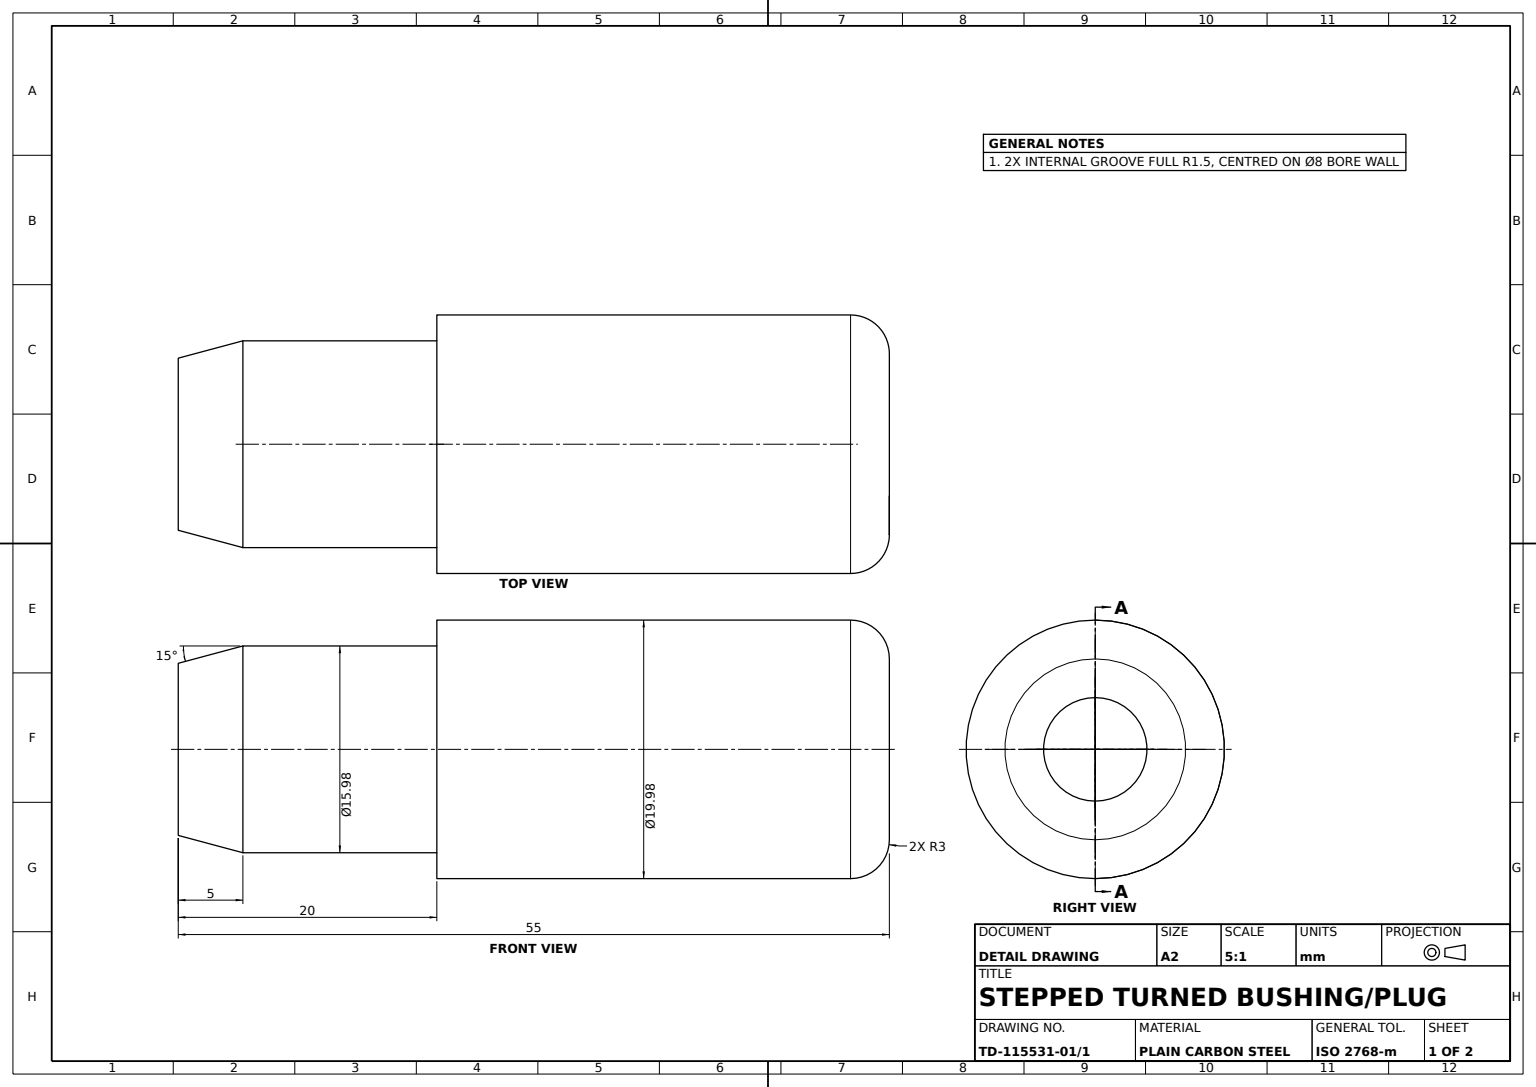
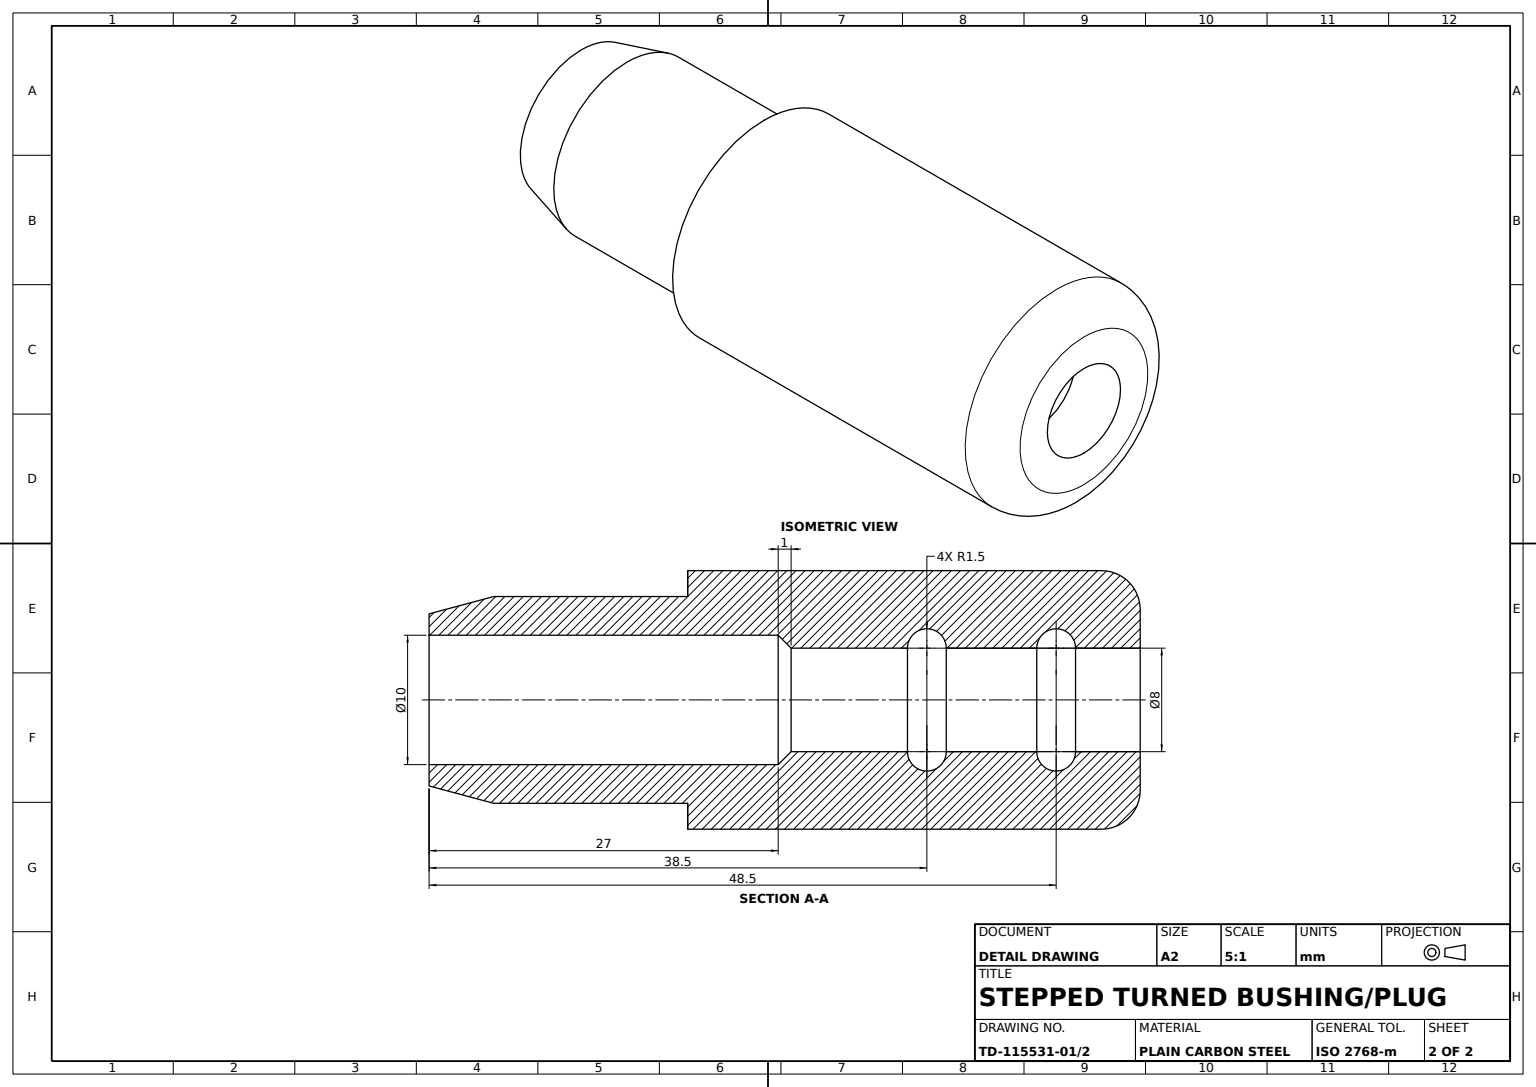
SolidWorks part; units mm, degrees
material "Plain Carbon Steel"
ref_plane "Front Plane" through (0, 0, 0) normal (0, 0, 1) x (1, 0, 0)
ref_plane "Top Plane" through (0, 0, 0) normal (0, 1, 0) x (1, 0, 0)
ref_plane "Right Plane" through (0, 0, 0) normal (1, 0, 0) x (0, 0, -1)
sketch "Pin Profile Sketch" plane through (0, 0, 0) normal (0, 0, 1) x (1, 0, 0)
  line L0 (0, 37.7176) -> (0, -40.5) construction
  line L1 (5, 0) -> (5, 27)
  line L2 (5, 27) -> (4, 28)
  line L3 (4, 28) -> (4, 37)
  line L4 (4, 40) -> (4, 47)
  line L5 (4, 50) -> (4, 55)
  line L6 (4, 55) -> (6.9897, 55)
  line L7 (9.9897, 52) -> (9.9897, 20)
  line L8 (9.9897, 20) -> (7.9897, 20)
  line L9 (7.9897, 20) -> (7.9897, 5)
  line L10 (7.9897, 5) -> (6.65, 0)
  line L11 (6.65, 0) -> (5, 0)
  arc A0 (4, 37) -> (4, 40) centre (4, 38.5) ccw
  arc A1 (4, 47) -> (4, 50) centre (4, 48.5) ccw
  arc A2 (6.9897, 55) -> (9.9897, 52) centre (6.9897, 52) cw
  dimension "D4" = 1.5
  dimension "D7" = 3
  dimension "D1" = 27
  dimension "D2" = 1
  dimension "D3" = 9
  dimension "D5" = 7
  dimension "D6" = 5
  dimension "D8" = 1.65
  dimension "D9" = 15
  dimension "D10" = 5
  dimension "D11" = 20
  dimension "D12" = 2
  dimension "D13" = 35
  dimension "D14" = 5
  dimension "D15" = 45
revolve "Pin Body Revolve" add sketch "Pin Profile Sketch" angle 360 about L0
